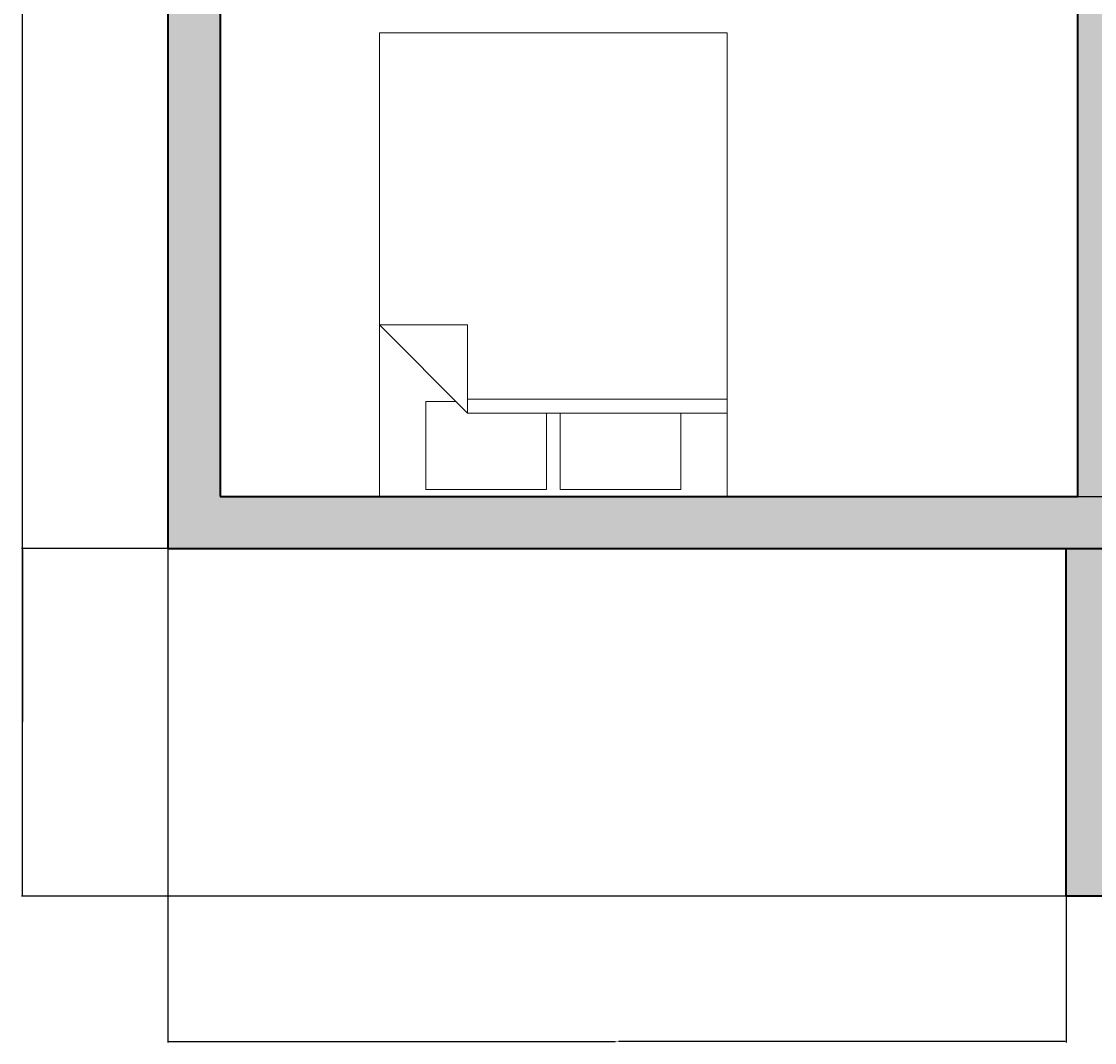
# Model space of a CAD drawing. Units: inches. Extents: x -12 to 539, y -477 to 51.
# Tile 1 of 6: x -12 to 173, y -477 to -301. Entities that reach past the tile are written whole.
import ezdxf

# ---------------------------------------------------------------- set-up
doc = ezdxf.new("R2010")
doc.units = ezdxf.units.IN
doc.header["$MEASUREMENT"] = 0
for name, color, linetype, lineweight in [('A-ANNO-DIMS', 2, 'Continuous', 18), ('A-FURN', 8, 'Continuous', 18), ('A-WALL', 7, 'Continuous', 35)]:
    doc.layers.add(name, color=color, linetype=linetype, lineweight=lineweight)
doc.layers.add('A-WALL-PATT', color=252, linetype='Continuous', lineweight=13, true_color=0x939598)
doc.styles.get("Standard").update_dxf_attribs({"font": 'arial.ttf'})
doc.dimstyles.get("Standard").update_dxf_attribs({"dimtxt": 0.18, "dimasz": 0.18, "dimexe": 0.18, "dimexo": 0.0625, "dimgap": 0.09, "dimtad": 0, "dimtih": 1, "dimtoh": 1, "dimdec": 0, "dimzin": 0, "dimdsep": 46, "dimlunit": 3, "dimtxsty": 'Standard', "dimcen": 0.09, "dimadec": 0, "dimazin": 0, "dimtfac": 1, "dimtdec": 0, "dimtofl": 0, "dimtmove": 0, "dimatfit": 3, "dimfxl": 1, "dimtolj": 1, "dimtzin": 0, "dimarcsym": 0})

# ---------------------------------------------------------------- blocks, each defined once
blk = doc.blocks.new('Bed - Queen')
for p, q in [((0, -80.00003), (0, 0)), ((0, 0), (59.99999, 0)), ((59.99999, 0), (59.99999, -80.00003)), ((7.99999, -1.2), (28.79998, -1.2)), ((7.99999, -14.4), (7.99999, -1.2)), ((28.79998, -1.2), (28.79998, -14.4)), ((31.19999, -1.2), (51.99999, -1.2)), ((31.19999, -14.4), (31.19999, -1.2)), ((51.99999, -1.2), (51.99999, -16.4)), ((0, -14.4), (44.8, -14.4)), ((59.99999, -29.6), (44.8, -14.4)), ((44.8, -14.4), (44.8, -29.6)), ((51.99999, -16.4), (46.79936, -16.4)), ((44.8, -16.8), (0, -16.8)), ((44.8, -29.6), (59.99999, -29.6)), ((59.99999, -80.00003), (0, -80.00003))]:
    blk.add_line(p, q)
blk = doc.blocks.new('*D38')
at = {"layer": 'A-ANNO-DIMS', "color": 0, "lineweight": -2, "transparency": 16777216}
for p, q in [((13.04, 26.01), (-12.14, 26.01)), ((-11.96, 25.83), (-11.96, -212.81)), ((-11.96, -451.81), (-11.96, -213.17)), ((168.04, -451.99), (-12.14, -451.99))]:
    blk.add_line(p, q, dxfattribs=at)
at = {"layer": 'A-ANNO-DIMS', "color": 0, "transparency": 16777216}
for points in [[(-11.99, 25.83), (-11.93, 25.83), (-11.96, 26.01)], [(-11.99, -451.81), (-11.93, -451.81), (-11.96, -451.99)]]:
    blk.add_solid(points, dxfattribs=at)
at = {"layer": 'Defpoints', "color": 0, "transparency": 16777216}
for p in [(13.1, 26.01), (-11.96, -451.99), (168.1, -451.99)]:
    blk.add_point(p, dxfattribs=at)
at = {"layer": 'A-ANNO-DIMS', "color": 0, "transparency": 16777216, "insert": (-11.96, -212.99), "char_height": 0.18, "attachment_point": 5}
blk.add_mtext('\\A1;478', dxfattribs=at)
blk = doc.blocks.new('*D41')
at = {"layer": 'A-ANNO-DIMS', "color": 0, "lineweight": -2, "transparency": 16777216}
for p, q in [((13.1, -392.05), (13.1, -477.23)), ((168.1, -392.05), (168.1, -477.23)), ((13.28, -477.05), (90.32, -477.05)), ((167.92, -477.05), (90.88, -477.05))]:
    blk.add_line(p, q, dxfattribs=at)
at = {"layer": 'A-ANNO-DIMS', "color": 0, "transparency": 16777216}
for points in [[(13.28, -477.02), (13.28, -477.08), (13.1, -477.05)], [(167.92, -477.02), (167.92, -477.08), (168.1, -477.05)]]:
    blk.add_solid(points, dxfattribs=at)
at = {"layer": 'Defpoints', "color": 0, "transparency": 16777216}
for p in [(13.1, -391.99), (168.1, -391.99), (168.1, -477.05)]:
    blk.add_point(p, dxfattribs=at)
at = {"layer": 'A-ANNO-DIMS', "color": 0, "transparency": 16777216, "insert": (90.6, -477.05), "char_height": 0.18, "attachment_point": 5}
blk.add_mtext('\\A1;155', dxfattribs=at)
blk = doc.blocks.new('*D43')
at = {"layer": 'A-ANNO-DIMS', "color": 0, "lineweight": -2, "transparency": 16777216}
for p, q in [((168.04, -391.99), (-12.14, -391.99)), ((-11.96, -392.17), (-11.96, -421.81)), ((-11.96, -451.81), (-11.96, -422.17)), ((168.04, -451.99), (-12.14, -451.99))]:
    blk.add_line(p, q, dxfattribs=at)
at = {"layer": 'A-ANNO-DIMS', "color": 0, "transparency": 16777216}
for points in [[(-11.99, -392.17), (-11.93, -392.17), (-11.96, -391.99)], [(-11.99, -451.81), (-11.93, -451.81), (-11.96, -451.99)]]:
    blk.add_solid(points, dxfattribs=at)
at = {"layer": 'Defpoints', "color": 0, "transparency": 16777216}
for p in [(-11.96, -391.99), (168.1, -391.99), (168.1, -451.99)]:
    blk.add_point(p, dxfattribs=at)
at = {"layer": 'A-ANNO-DIMS', "color": 0, "transparency": 16777216, "insert": (-11.96, -421.99), "char_height": 0.18, "attachment_point": 5}
blk.add_mtext('\\A1;60', dxfattribs=at)
blk = doc.blocks.new('*D45')
at = {"layer": 'A-ANNO-DIMS', "color": 0, "lineweight": -2, "transparency": 16777216}
for p, q in [((22.17, -382.99), (539.23, -382.99)), ((539.05, -383.17), (539.05, -387.31)), ((539.05, -391.81), (539.05, -387.67)), ((13.17, -391.99), (539.23, -391.99))]:
    blk.add_line(p, q, dxfattribs=at)
at = {"layer": 'A-ANNO-DIMS', "color": 0, "transparency": 16777216}
for points in [[(539.02, -383.17), (539.08, -383.17), (539.05, -382.99)], [(539.02, -391.81), (539.08, -391.81), (539.05, -391.99)]]:
    blk.add_solid(points, dxfattribs=at)
at = {"layer": 'Defpoints', "color": 0, "transparency": 16777216}
for p in [(22.1, -382.99), (539.05, -382.99), (13.1, -391.99)]:
    blk.add_point(p, dxfattribs=at)
at = {"layer": 'A-ANNO-DIMS', "color": 0, "transparency": 16777216, "insert": (539.05, -387.49), "char_height": 0.18, "attachment_point": 5}
blk.add_mtext('\\A1;9', dxfattribs=at)

msp = doc.modelspace()

# ---------------------------------------------------------------- hatches: boundary and pattern name
at = {"layer": 'A-WALL-PATT'}
h = msp.add_hatch(color=256, dxfattribs=at)
h.dxf.hatch_style = 1
h.paths.add_polyline_path([(267.143, 26.0124), (13.1031, 26.0124), (13.1031, -391.9876), (177.1031, -391.9876), (177.1031, -346.9876), (307.7315, -346.9876), (321.1031, -346.9876), (321.1031, -389.9876), (469.1031, -389.9876), (469.1031, 26.0124), (302.7142, 26.0124), (302.7142, 17.0124), (321.1031, 17.0124), (321.1031, -131.577, -0.04877504), (328.1031, -132.2621), (328.1031, 17.0124), (460.1031, 17.0124), (460.1031, -124.9876), (382.1031, -124.9876), (379.1031, -124.9876), (379.1031, -131.5624), (382.1031, -131.5624), (382.1031, -127.9876), (460.1031, -127.9876), (460.1031, -153.7747), (460.1031, -199.9876), (382.1031, -199.9876), (382.1031, -167.7132), (379.1031, -167.7132), (379.1031, -199.9876), (328.1031, -199.9876), (328.1031, -167.7132), (321.1031, -167.7132), (321.1031, -206.9876), (460.1031, -206.9876), (460.1031, -323.9876), (388.677, -323.9876, -0.02504709), (388.5266, -326.9876), (460.1031, -326.9876), (460.1031, -380.9876), (328.1031, -380.9876), (328.1031, -326.9876), (358.677, -326.9876), (358.677, -323.9876), (328.1031, -323.9876), (328.1031, -296.9562), (321.1031, -296.9562), (321.1031, -339.9876), (307.7315, -339.9876), (177.1031, -339.9876), (177.1031, -250.9876), (244.0259, -250.9876), (244.0259, -243.9876), (163.7315, -243.9876), (163.7315, -250.9876), (170.1031, -250.9876), (170.1031, -382.9876), (22.1031, -382.9876), (22.1031, -250.9876), (41.3871, -250.9876, -0.06888376), (40.8612, -243.9876), (22.1031, -243.9876), (22.1031, -183.9876), (118.1031, -183.9876), (118.1031, -243.9876), (71.6031, -243.9876), (71.6031, -250.9876), (128.4772, -250.9876, -0.04900189), (127.7315, -243.9876), (121.1031, -243.9876), (121.1031, -183.9876), (121.1031, -120.9876), (118.1031, -120.9876), (118.1031, -180.9876), (22.1031, -180.9876), (22.1031, -120.9876), (49.0045, -120.9876, -0.07000725), (46.9084, -111.9876), (46.1728, -111.9876), (22.1031, -111.9876), (22.1031, 17.0124), (170.1031, 17.0124), (170.1031, -120.9876), (177.1031, -120.9876), (177.1031, 17.0124), (268.2584, 17.0124, -0.0639977)])
h.paths.add_polyline_path([(513.9866, -124.9876), (469.1031, -124.9876), (469.1031, -127.9876), (510.9866, -127.9876), (510.9866, -259.2045), (469.1031, -259.2045), (469.1031, -262.2045), (513.9866, -262.2045)])
h.paths.add_polyline_path([(351.8833, -206.9876), (348.8833, -206.9876), (348.8833, -253.547), (328.1031, -253.547), (321.1031, -253.547), (321.1031, -256.547), (328.1031, -256.547), (351.8833, -256.547)], flags=17)
h.paths.add_polyline_path([(330.1031, -389.9876), (321.1031, -389.9876), (321.1031, -442.9876), (177.1031, -442.9876), (177.1031, -391.9876), (168.1031, -391.9876), (168.1031, -451.9876), (330.1031, -451.9876)])
h.paths.add_polyline_path([(414.1504, -177.6962), (465.5248, -177.6962), (465.5248, -164.7437), (414.1504, -164.7437)], flags=25)

# ---------------------------------------------------------------- linework, layer by layer
at = {"layer": 'A-WALL'}
for p, q in [((13.1031, 26.0124), (13.1031, -391.9876)), ((13.1031, -250.9876), (13.1031, -382.9876)), ((22.1031, -250.9876), (22.1031, -382.9876)), ((170.1031, -382.9876), (170.1031, -250.9876)), ((22.1031, -382.9876), (170.1031, -382.9876)), ((13.1031, -391.9876), (177.1031, -391.9876)), ((168.1031, -451.9876), (168.1031, -391.9876)), ((330.1031, -451.9876), (168.1031, -451.9876))]:
    msp.add_line(p, q, dxfattribs=at)

# ---------------------------------------------------------------- block references
at = {"layer": 'A-FURN', "rotation": 180}
msp.add_blockref('Bed - Queen', (109.6235, -382.9876), dxfattribs=at)

# ---------------------------------------------------------------- dimensions: what is measured, and where the dimension line sits
at = {"layer": 'A-ANNO-DIMS'}
for base, p1, p2, picture, middle in [((-11.9569, -451.9876), (13.1031, 26.0124), (168.1031, -451.9876), '*D38', (-11.9569, -212.9876)), ((539.0466, -382.9876), (13.1031, -391.9876), (22.1031, -382.9876), '*D45', (539.0466, -387.4876)), ((-11.9569, -391.9876), (168.1031, -451.9876), (168.1031, -391.9876), '*D43', (-11.9569, -421.9876))]:
    dim = msp.add_linear_dim(base=base, p1=p1, p2=p2, angle=90, dimstyle='Standard', override={"dimdec": 0, "dimlfac": 1, "dimrnd": 0, "dimzin": 0, "dimdsep": 46, "dimlunit": 2}, dxfattribs=at)
    dim.commit()
    dim.dimension.update_dxf_attribs({"geometry": picture, "text_midpoint": middle})
dim = msp.add_linear_dim(base=(168.1031, -477.0476), p1=(13.1031, -391.9876), p2=(168.1031, -391.9876), dimstyle='Standard', override={"dimdec": 0, "dimlfac": 1, "dimrnd": 0, "dimzin": 0, "dimdsep": 46, "dimlunit": 2}, dxfattribs=at)
dim.commit()
dim.dimension.update_dxf_attribs({"geometry": '*D41', "text_midpoint": (90.6031, -477.0476)})

doc.saveas('drawing.dxf')
